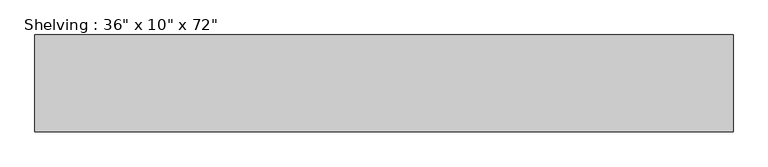
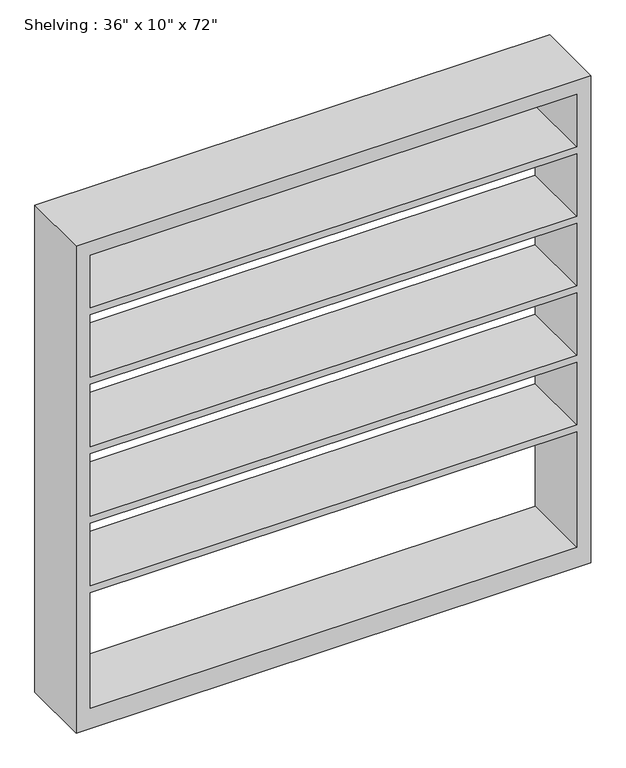
"""IFC4 building model written with IfcOpenShell, lengths in millimetres: furniture geometry."""

from ifc_helpers import new_model, si_unit, frame, origin, place, context, project, spatial, polyline, outline, extrude, source, transform, mapped, element, save


def furniture_c6fa4874(model_context):
    return source(origin(), model_context, "Body", "SweptSolid", [
        extrude(outline(polyline([(0.0, 914.4), (1828.8, 914.4), (1828.8, -914.4), (0.0, -914.4), (0.0, 914.4)]), holes=[polyline([(1778.0, 863.6), (1580.2428571, 863.6), (1580.2428571, -863.6), (1778.0, -863.6), (1778.0, 863.6)]), polyline([(76.2, 863.6), (76.2, -863.6), (509.8142857, -863.6), (509.8142857, 863.6), (76.2, 863.6)]), polyline([(1057.7285714, -863.6), (1293.5857143, -863.6), (1293.5857143, 863.6), (1057.7285714, 863.6), (1057.7285714, -863.6)]), polyline([(1554.8428571, 863.6), (1318.9857143, 863.6), (1318.9857143, -863.6), (1554.8428571, -863.6), (1554.8428571, 863.6)]), polyline([(1032.3285714, 863.6), (796.4714286, 863.6), (796.4714286, -863.6), (1032.3285714, -863.6), (1032.3285714, 863.6)]), polyline([(771.0714286, 863.6), (535.2142857, 863.6), (535.2142857, -863.6), (771.0714286, -863.6), (771.0714286, 863.6)])]), frame((0.0, -431.8, 0.0), z_axis=(0.0, 1.0, 0.0), x_axis=(0.0, 0.0, 1.0)), (0.0, 0.0, 1.0), 254.0),
    ])


if __name__ == "__main__":
    model = new_model("IFC4")
    model_context = context("Model", 3, world=origin())
    ifc_project = project(units=[si_unit("LENGTHUNIT", "METRE", prefix="MILLI")], contexts=[model_context])
    site = spatial("IfcSite", under=ifc_project)
    building = spatial("IfcBuilding", under=site)
    placement = place(None, origin())
    furniture_shape = furniture_c6fa4874(model_context)
    element("IfcFurniture", 1, ObjectType="Shelving : 36\" x 10\" x 72\"", at=placement, inside=building, context=model_context, shape_type="MappedRepresentation", body=[
        mapped(furniture_shape, transform((0.0, 0.0, 0.0), x_axis=(1.0, 0.0, 0.0), y_axis=(0.0, 1.0, 0.0), z_axis=(0.0, 0.0, 1.0))),
    ])
    save(model, "model.ifc")

# Revit data of these elements
# Type "Shelving : 36\" x 10\" x 72\""
#   Assembly Code = "E2020200"
#   Depth = 0' - 10"
#   Height = 6' - 0"
#   Width = 6' - 0"
#   Shelving Unit Material = Birch
#   Default Elevation = 0
# Element 1 (IfcFurniture, "Shelving : 36\" x 10\" x 72\"")
#   Materials on its faces: "Birch"
# Materials
#   "Birch": class "Wood", colour RGB 224 178 126, transparency 0, Description = "Betula Alleghaniensis", Cost = 0
